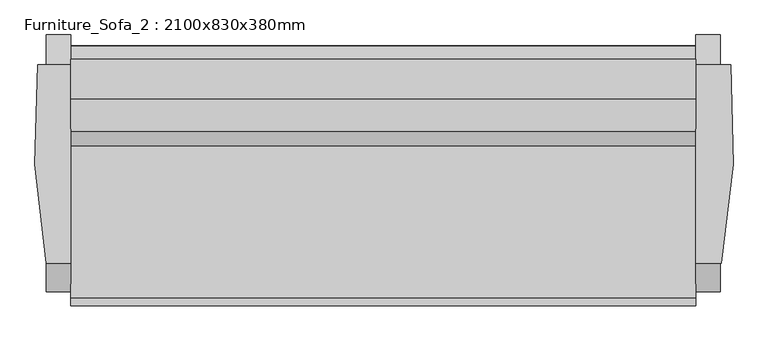
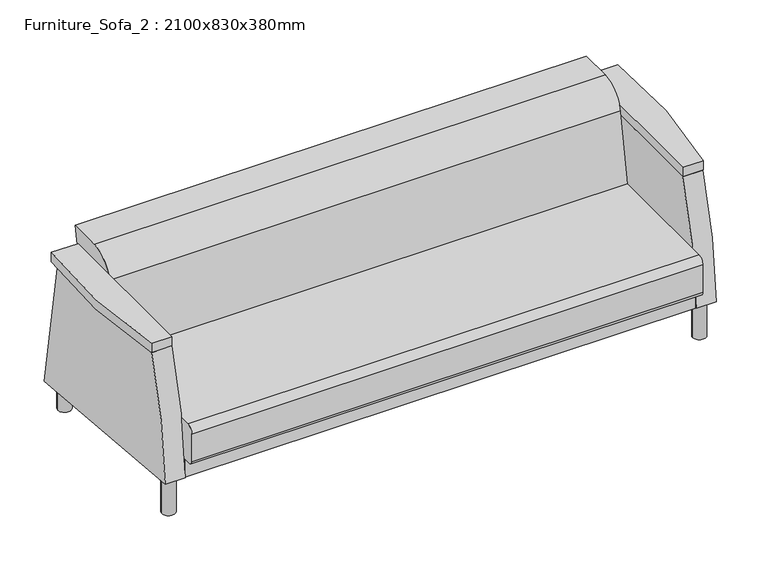
"""IFC4 building model written with IfcOpenShell, lengths in millimetres: furniture geometry, Furniture_Sofa_2 : 2100x830x380mm."""

from ifc_helpers import new_model, si_unit, point, frame, frame_2d, origin, origin_with_axes, place, context, project, spatial, polyline, circle_curve, trimmed, segment, composite_curve, outline, extrude, source, transform, mapped, element, save


def furniture_sofa_2_2100x830x380mm_2cdf16e3(model_context):
    return source(origin(), model_context, "Body", "SweptSolid", [
        extrude(outline(composite_curve([segment(trimmed(circle_curve(frame_2d((-116.5901639, 351.2509954)), 25.4), [point((-141.9901639, 351.2509954))], [point((-116.5901639, 376.6509954))], False, "CARTESIAN"), True, "CONTINUOUS"), segment(polyline([(-116.5901639, 376.6509954), (355.3895541, 376.6509954), (402.1988177, 642.1195211)]), True, "CONTINUOUS"), segment(trimmed(circle_curve(frame_2d((502.2552854, 624.4768662)), 101.6), [point((402.1988177, 642.1195211))], [point((502.2552854, 726.0768662))], False, "CARTESIAN"), True, "CONTINUOUS"), segment(polyline([(502.2552854, 726.0768662), (626.3344485, 726.0768662), (609.5377828, 620.1719187), (667.6541767, 224.2509954), (-126.1151639, 224.2509954)]), True, "CONTINUOUS"), segment(trimmed(circle_curve(frame_2d((-126.1151639, 240.1259954)), 15.875), [point((-126.1151639, 224.2509954))], [point((-141.9901639, 240.1259954))], False, "CARTESIAN"), True, "CONTINUOUS"), segment(polyline([(-141.9901639, 240.1259954), (-141.9901639, 351.2509954)]), True, "CONTINUOUS")], self_intersect=False)), frame((-695.19375, 0.0, 0.0), z_axis=(1.0, 0.0, 0.0), x_axis=(0.0, 1.0, 0.0)), (0.0, 0.0, 1.0), 1947.6),
        extrude(outline(composite_curve([segment(polyline([(701.7619204, 79.3588346), (-97.7900405, 149.3105671)]), True, "CONTINUOUS"), segment(trimmed(circle_curve(frame_2d((1499.9783711, 99.5888442)), 1598.5418814), [point((-97.7900405, 149.3105671))], [point((-9.3943348, 626.0203985))], False, "CARTESIAN"), True, "CONTINUOUS"), segment(polyline([(-9.3943348, 626.0203985), (608.6917937, 626.0203985), (701.7619204, 79.3588346)]), True, "CONTINUOUS")], self_intersect=False)), frame((1252.40625, 0.0, 0.0), z_axis=(1.0, 0.0, 0.0), x_axis=(0.0, 1.0, 0.0)), (0.0, 0.0, 1.0), 76.2),
        extrude(outline(composite_curve([segment(polyline([(-9.3943348, 626.0203985), (608.6917937, 626.0203985), (701.7619204, 79.3588346), (-97.7900405, 149.3105671)]), True, "CONTINUOUS"), segment(trimmed(circle_curve(frame_2d((1499.9783711, 99.5888442)), 1598.5418814), [point((-97.7900405, 149.3105671))], [point((-9.3943348, 626.0203985))], False, "CARTESIAN"), True, "CONTINUOUS")], self_intersect=False)), frame((-771.39375, 0.0, 0.0), z_axis=(1.0, 0.0, 0.0), x_axis=(0.0, 1.0, 0.0)), (0.0, 0.0, 1.0), 76.2),
        extrude(outline(polyline([(1252.40625, 668.3047863), (1252.40625, -93.6952137), (-695.19375, -93.6952137), (-695.19375, 668.3047863), (1252.40625, 668.3047863)])), frame((0.0, 0.0, 148.0509954), z_axis=(0.0, 0.0, 1.0), x_axis=(1.0, 0.0, 0.0)), (0.0, 0.0, 1.0), 76.2),
        extrude(outline(composite_curve([segment(trimmed(circle_curve(frame_2d((-733.29375, -53.0901639)), 25.4), [point((-758.69375, -53.0901639))], [point((-707.89375, -53.0901639))], False, "CARTESIAN"), True, "CONTINUOUS"), segment(trimmed(circle_curve(frame_2d((-733.29375, -53.0901639)), 25.4), [point((-707.89375, -53.0901639))], [point((-758.69375, -53.0901639))], False, "CARTESIAN"), True, "CONTINUOUS")], self_intersect=False)), origin_with_axes(), (0.0, 0.0, 1.0), 148.43125),
        extrude(outline(composite_curve([segment(trimmed(circle_curve(frame_2d((-733.29375, 632.7098361)), 25.4), [point((-758.69375, 632.7098361))], [point((-707.89375, 632.7098361))], False, "CARTESIAN"), True, "CONTINUOUS"), segment(trimmed(circle_curve(frame_2d((-733.29375, 632.7098361)), 25.4), [point((-707.89375, 632.7098361))], [point((-758.69375, 632.7098361))], False, "CARTESIAN"), True, "CONTINUOUS")], self_intersect=False)), origin_with_axes(), (0.0, 0.0, 1.0), 148.43125),
        extrude(outline(composite_curve([segment(trimmed(circle_curve(frame_2d((1290.50625, 632.7098361)), 25.4), [point((1265.10625, 632.7098361))], [point((1315.90625, 632.7098361))], False, "CARTESIAN"), True, "CONTINUOUS"), segment(trimmed(circle_curve(frame_2d((1290.50625, 632.7098361)), 25.4), [point((1315.90625, 632.7098361))], [point((1265.10625, 632.7098361))], False, "CARTESIAN"), True, "CONTINUOUS")], self_intersect=False)), origin_with_axes(), (0.0, 0.0, 1.0), 148.43125),
        extrude(outline(composite_curve([segment(trimmed(circle_curve(frame_2d((1290.50625, -53.0901639)), 25.4), [point((1265.10625, -53.0901639))], [point((1315.90625, -53.0901639))], False, "CARTESIAN"), True, "CONTINUOUS"), segment(trimmed(circle_curve(frame_2d((1290.50625, -53.0901639)), 25.4), [point((1315.90625, -53.0901639))], [point((1265.10625, -53.0901639))], False, "CARTESIAN"), True, "CONTINUOUS")], self_intersect=False)), origin_with_axes(), (0.0, 0.0, 1.0), 148.43125),
        extrude(outline(composite_curve([segment(polyline([(-695.19375, -9.3943348), (-771.39375, -9.3943348)]), True, "CONTINUOUS"), segment(trimmed(circle_curve(frame_2d((1362.7527561, 387.8725201)), 2170.8068232), [point((-771.39375, -9.3943348))], [point((-796.79375, 608.6917935))], False, "CARTESIAN"), True, "CONTINUOUS"), segment(polyline([(-796.79375, 608.6917935), (-695.19375, 608.6917935), (-695.19375, -9.3943348)]), True, "CONTINUOUS")], self_intersect=False)), frame((0.0, 0.0, 626.0203985), z_axis=(0.0, 0.0, 1.0), x_axis=(1.0, 0.0, 0.0)), (0.0, 0.0, 1.0), 38.1),
        extrude(outline(composite_curve([segment(polyline([(1252.40625, -9.3943348), (1252.40625, 608.9395268), (1361.0864453, 608.9395268)]), True, "CONTINUOUS"), segment(trimmed(circle_curve(frame_2d((-804.5771494, 405.3576786)), 2175.2113402), [point((1361.0864453, 608.9395268))], [point((1330.7273117, -9.3943348))], False, "CARTESIAN"), True, "CONTINUOUS"), segment(polyline([(1330.7273117, -9.3943348), (1252.40625, -9.3943348)]), True, "CONTINUOUS")], self_intersect=False)), frame((0.0, 0.0, 626.0203985), z_axis=(0.0, 0.0, 1.0), x_axis=(1.0, 0.0, 0.0)), (0.0, 0.0, 1.0), 38.1),
    ])


if __name__ == "__main__":
    model = new_model("IFC4")
    model_context = context("Model", 3, world=origin())
    ifc_project = project(units=[si_unit("LENGTHUNIT", "METRE", prefix="MILLI")], contexts=[model_context])
    site = spatial("IfcSite", under=ifc_project)
    building = spatial("IfcBuilding", under=site)
    placement = place(None, origin())
    furniture_sofa_2_2100x830x380mm_shape = furniture_sofa_2_2100x830x380mm_2cdf16e3(model_context)
    element("IfcFurniture", 1, ObjectType="Furniture_Sofa_2 : 2100x830x380mm", at=placement, inside=building, context=model_context, shape_type="MappedRepresentation", body=[
        mapped(furniture_sofa_2_2100x830x380mm_shape, transform((0.0, 0.0, 0.0), x_axis=(1.0, 0.0, 0.0), y_axis=(0.0, 1.0, 0.0), z_axis=(0.0, 0.0, 1.0))),
    ])
    save(model, "model.ifc")

# Revit data of these elements
# Type "Furniture_Sofa_2 : 2100x830x380mm"
#   Keynote = "N"
#   Length = 6' - 10.67717"
#   Material Sofa = Textile - Linen, Smooth
#   Material Frame = Metal - Chrome
#   Default Elevation = 0
# Element 1 (IfcFurniture, "Furniture_Sofa_2 : 2100x830x380mm")
#   Materials on its faces: "Textile - Linen, Smooth", "Metal - Chrome"
# Materials
#   "Textile - Linen, Smooth": class "Fabric", colour RGB 249 239 230, transparency 0
#   "Metal - Chrome": class "Metal", colour RGB 17 17 17, transparency 0
